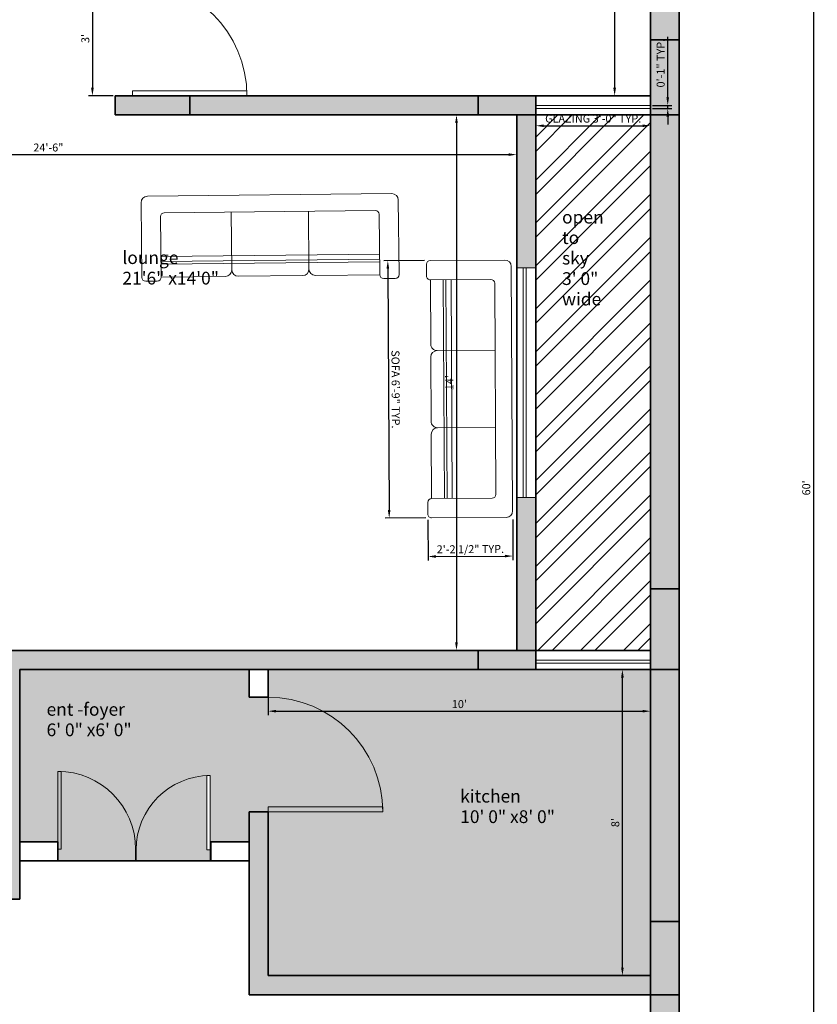
# Model space of a CAD drawing. Units: inches. Extents: x 2369 to 4208, y 1650 to 4492.
# Tile 4 of 6: x 2570 to 2820, y 1948 to 2257. Entities that reach past the tile are written whole.
import ezdxf

# ---------------------------------------------------------------- set-up
doc = ezdxf.new("R2010")
doc.units = ezdxf.units.IN
for name, color, linetype, lineweight in [('A-ANNO-DIMS', 2, 'Continuous', 13), ('A-AREA-IDEN', 7, 'Continuous', 18), ('A-COLS', 7, 'Continuous', 35), ('A-COLS-PATT', 7, 'Continuous', 13), ('A-DOOR', 4, 'Continuous', 18), ('A-FLOR-PATT', 9, 'Continuous', 13), ('A-FURN', 8, 'Continuous', 18), ('A-GLAZ', 4, 'Continuous', 18), ('A-WALL', 7, 'Continuous', 35), ('A-WALL-PATT', 252, 'Continuous', 13)]:
    doc.layers.add(name, color=color, linetype=linetype, lineweight=lineweight)
doc.styles.get("Standard").update_dxf_attribs({"font": 'arial.ttf'})
doc.dimstyles.new('Copy of ISO-25', dxfattribs={"dimtxt": 2.5, "dimasz": 2.5, "dimexe": 1.25, "dimexo": 0.625, "dimtad": 1, "dimdec": 1, "dimlunit": 4, "dimtxsty": 'Standard', "dimcen": 2.5, "dimadec": 0, "dimazin": 0, "dimtfac": 1, "dimtdec": 1, "dimtmove": 0, "dimatfit": 3, "dimfxl": 1, "dimarcsym": 0})

# ---------------------------------------------------------------- blocks, each defined once
blk = doc.blocks.new('*U5')
for p, q in [((0, 0), (0, -6)), ((-40, 0), (-40, -6))]:
    blk.add_line(p, q)
blk.add_lwpolyline([(0, 0), (0, 40), (-1.75, 40), (-1.75, 0)], close=True)
blk.add_arc((0, 0), 40, 90, 180)
blk = doc.blocks.new('*U4')
for p, q in [((-40, 0), (-40, 6)), ((0, 0), (0, 6))]:
    blk.add_line(p, q)
blk.add_lwpolyline([(0, 0), (0, -40), (-1.75, -40), (-1.75, 0)], close=True)
blk.add_arc((0, 0), 40, 180, 270)
blk = doc.blocks.new('*U2')
for p, q in [((0, 0), (0, -6)), ((40, 0), (40, -6))]:
    blk.add_line(p, q)
blk.add_lwpolyline([(0, 0), (0, 40), (1.75, 40), (1.75, 0)], close=True)
blk.add_arc((0, 0), 40, 0, 90)
blk = doc.blocks.new('*U3')
for p, q in [((0, 0), (0, -6)), ((-40, 0), (-40, -6))]:
    blk.add_line(p, q)
blk.add_lwpolyline([(0, 0), (0, 40), (-1.75, 40), (-1.75, 0)], close=True)
blk.add_arc((0, 0), 40, 90, 180)
blk = doc.blocks.new('*D8')
at = {"layer": 'A-ANNO-DIMS', "color": 0, "lineweight": -2, "transparency": 16777216}
for p, q in [((2777.53, 2469.98), (2820.25, 2469.98)), ((2819, 2467.48), (2819, 1752.48)), ((2777.53, 1749.98), (2820.25, 1749.98))]:
    blk.add_line(p, q, dxfattribs=at)
at = {"layer": 'A-ANNO-DIMS', "color": 0, "transparency": 16777216}
for points in [[(2818.58, 2467.48), (2819.41, 2467.48), (2819, 2469.98)], [(2818.58, 1752.48), (2819.41, 1752.48), (2819, 1749.98)]]:
    blk.add_solid(points, dxfattribs=at)
at = {"layer": 'Defpoints', "color": 0, "transparency": 16777216}
for p in [(2776.9, 2469.98), (2776.9, 1749.98), (2819, 1749.98)]:
    blk.add_point(p, dxfattribs=at)
at = {"layer": 'A-ANNO-DIMS', "color": 0, "transparency": 16777216, "insert": (2817.1, 2109.98), "char_height": 2.5, "attachment_point": 5, "rotation": 90}
blk.add_mtext("60'", dxfattribs=at)
blk = doc.blocks.new('*D22')
at = {"layer": 'A-ANNO-DIMS', "color": 0, "lineweight": -2, "transparency": 16777216}
for p, q in [((2767.28, 2394.98), (2755.38, 2394.98)), ((2756.63, 2392.48), (2756.63, 2235.48)), ((2767.28, 2232.98), (2755.38, 2232.98))]:
    blk.add_line(p, q, dxfattribs=at)
at = {"layer": 'A-ANNO-DIMS', "color": 0, "transparency": 16777216}
for points in [[(2756.21, 2392.48), (2757.05, 2392.48), (2756.63, 2394.98)], [(2756.21, 2235.48), (2757.05, 2235.48), (2756.63, 2232.98)]]:
    blk.add_solid(points, dxfattribs=at)
at = {"layer": 'Defpoints', "color": 0, "transparency": 16777216}
for p in [(2767.9, 2394.98), (2756.63, 2232.98), (2767.9, 2232.98)]:
    blk.add_point(p, dxfattribs=at)
at = {"layer": 'A-ANNO-DIMS', "color": 0, "transparency": 16777216, "insert": (2754.73, 2313.98), "char_height": 2.5, "attachment_point": 5, "rotation": 90}
blk.add_mtext('13\'-6"', dxfattribs=at)
blk = doc.blocks.new('*D27')
at = {"layer": 'A-ANNO-DIMS', "color": 0, "lineweight": -2, "transparency": 16777216}
for p, q in [((2431.9, 2226.35), (2431.9, 2213.28)), ((2725.9, 2226.35), (2725.9, 2213.28)), ((2434.4, 2214.53), (2723.4, 2214.53))]:
    blk.add_line(p, q, dxfattribs=at)
at = {"layer": 'A-ANNO-DIMS', "color": 0, "transparency": 16777216}
for points in [[(2434.4, 2214.94), (2434.4, 2214.11), (2431.9, 2214.53)], [(2723.4, 2214.94), (2723.4, 2214.11), (2725.9, 2214.53)]]:
    blk.add_solid(points, dxfattribs=at)
at = {"layer": 'Defpoints', "color": 0, "transparency": 16777216}
for p in [(2431.9, 2226.98), (2725.9, 2226.98), (2725.9, 2214.53)]:
    blk.add_point(p, dxfattribs=at)
at = {"layer": 'A-ANNO-DIMS', "color": 0, "transparency": 16777216, "insert": (2578.9, 2216.43), "char_height": 2.5, "attachment_point": 5}
blk.add_mtext('24\'-6"', dxfattribs=at)
blk = doc.blocks.new('*D28')
at = {"layer": 'A-ANNO-DIMS', "color": 0, "lineweight": -2, "transparency": 16777216}
for p, q in [((2725.28, 2226.98), (2705.75, 2226.98)), ((2707, 2224.48), (2707, 2061.48)), ((2725.28, 2058.98), (2705.75, 2058.98))]:
    blk.add_line(p, q, dxfattribs=at)
at = {"layer": 'A-ANNO-DIMS', "color": 0, "transparency": 16777216}
for points in [[(2706.58, 2224.48), (2707.41, 2224.48), (2707, 2226.98)], [(2706.58, 2061.48), (2707.41, 2061.48), (2707, 2058.98)]]:
    blk.add_solid(points, dxfattribs=at)
at = {"layer": 'Defpoints', "color": 0, "transparency": 16777216}
for p in [(2725.9, 2226.98), (2707, 2058.98), (2725.9, 2058.98)]:
    blk.add_point(p, dxfattribs=at)
at = {"layer": 'A-ANNO-DIMS', "color": 0, "transparency": 16777216, "insert": (2705.12, 2142.98), "char_height": 2.5, "attachment_point": 5, "rotation": 90}
blk.add_mtext("14'", dxfattribs=at)
blk = doc.blocks.new('*D31')
at = {"layer": 'A-ANNO-DIMS', "color": 0, "lineweight": -2, "transparency": 16777216}
for p, q in [((2647.9, 2052.35), (2647.9, 2038.68)), ((2767.9, 2052.35), (2767.9, 2038.68)), ((2650.4, 2039.93), (2765.4, 2039.93))]:
    blk.add_line(p, q, dxfattribs=at)
at = {"layer": 'A-ANNO-DIMS', "color": 0, "transparency": 16777216}
for points in [[(2650.4, 2040.34), (2650.4, 2039.51), (2647.9, 2039.93)], [(2765.4, 2040.34), (2765.4, 2039.51), (2767.9, 2039.93)]]:
    blk.add_solid(points, dxfattribs=at)
at = {"layer": 'Defpoints', "color": 0, "transparency": 16777216}
for p in [(2647.9, 2052.98), (2767.9, 2052.98), (2767.9, 2039.93)]:
    blk.add_point(p, dxfattribs=at)
at = {"layer": 'A-ANNO-DIMS', "color": 0, "transparency": 16777216, "insert": (2707.9, 2041.83), "char_height": 2.5, "attachment_point": 5}
blk.add_mtext("10'", dxfattribs=at)
blk = doc.blocks.new('*D32')
at = {"layer": 'A-ANNO-DIMS', "color": 0, "lineweight": -2, "transparency": 16777216}
for p, q in [((2767.28, 2052.98), (2757.82, 2052.98)), ((2759.07, 1959.48), (2759.07, 2050.48)), ((2767.28, 1956.98), (2757.82, 1956.98))]:
    blk.add_line(p, q, dxfattribs=at)
at = {"layer": 'A-ANNO-DIMS', "color": 0, "transparency": 16777216}
for points in [[(2758.66, 2050.48), (2759.49, 2050.48), (2759.07, 2052.98)], [(2758.66, 1959.48), (2759.49, 1959.48), (2759.07, 1956.98)]]:
    blk.add_solid(points, dxfattribs=at)
at = {"layer": 'Defpoints', "color": 0, "transparency": 16777216}
for p in [(2759.07, 2052.98), (2767.9, 2052.98), (2767.9, 1956.98)]:
    blk.add_point(p, dxfattribs=at)
at = {"layer": 'A-ANNO-DIMS', "color": 0, "transparency": 16777216, "insert": (2757.17, 2004.98), "char_height": 2.5, "attachment_point": 5, "rotation": 90}
blk.add_mtext("8'", dxfattribs=at)
blk = doc.blocks.new('*D43')
at = {"layer": 'A-ANNO-DIMS', "color": 0, "lineweight": -2, "transparency": 16777216}
for p, q in [((2599.28, 2268.93), (2591.48, 2268.93)), ((2592.73, 2266.43), (2592.73, 2235.48)), ((2599.28, 2232.98), (2591.48, 2232.98))]:
    blk.add_line(p, q, dxfattribs=at)
at = {"layer": 'A-ANNO-DIMS', "color": 0, "transparency": 16777216}
for points in [[(2592.31, 2266.43), (2593.15, 2266.43), (2592.73, 2268.93)], [(2592.31, 2235.48), (2593.15, 2235.48), (2592.73, 2232.98)]]:
    blk.add_solid(points, dxfattribs=at)
at = {"layer": 'Defpoints', "color": 0, "transparency": 16777216}
for p in [(2599.9, 2268.93), (2592.73, 2232.98), (2599.9, 2232.98)]:
    blk.add_point(p, dxfattribs=at)
at = {"layer": 'A-ANNO-DIMS', "color": 0, "transparency": 16777216, "insert": (2590.83, 2250.95), "char_height": 2.5, "attachment_point": 5, "rotation": 90}
blk.add_mtext("3'", dxfattribs=at)
blk = doc.blocks.new('A$C05BA3A2B')
for p, q in [((0.05, 0.6596), (1.95, 0.6596)), ((0.05, 0.6596), (1.95, 0.6596)), ((0.05, 0.6596), (1.95, 0.6596)), ((0, 0.03), (0, 0.6096)), ((0, 0.03), (0, 0.6096)), ((0, 0.03), (0, 0.6096)), ((2, 0.6096), (2, 0.03)), ((2, 0.6096), (2, 0.03)), ((2, 0.6096), (2, 0.03)), ((0.15, 0.5), (0.15, 0.03)), ((0.15, 0.5), (0.15, 0.03)), ((0.15, 0.5), (0.15, 0.03)), ((1.82, 0.53), (0.18, 0.53)), ((1.82, 0.53), (0.18, 0.53)), ((1.82, 0.53), (0.18, 0.53)), ((0.7, 0.08), (0.7, 0.53)), ((0.7, 0.08), (0.7, 0.53)), ((0.7, 0.08), (0.7, 0.53)), ((1.3, 0.53), (1.3, 0.08)), ((1.3, 0.53), (1.3, 0.08)), ((1.3, 0.53), (1.3, 0.08)), ((1.85, 0.03), (1.85, 0.5)), ((1.85, 0.03), (1.85, 0.5)), ((1.85, 0.03), (1.85, 0.5)), ((1.85, 0.1908), (0.15, 0.1908)), ((1.85, 0.1908), (0.15, 0.1908)), ((1.85, 0.1908), (0.15, 0.1908)), ((1.85, 0.1508), (0.15, 0.1508)), ((1.85, 0.1508), (0.15, 0.1508)), ((1.85, 0.1508), (0.15, 0.1508)), ((1.85, 0.1308), (0.15, 0.1308)), ((1.85, 0.1308), (0.15, 0.1308)), ((1.85, 0.1308), (0.15, 0.1308)), ((0.12, 0), (0.03, 0)), ((0.12, 0), (0.03, 0)), ((0.12, 0), (0.03, 0)), ((0.65, 0.03), (0.15, 0.03)), ((0.65, 0.03), (0.15, 0.03)), ((0.65, 0.03), (0.15, 0.03)), ((1.25, 0.03), (0.75, 0.03)), ((1.25, 0.03), (0.75, 0.03)), ((1.25, 0.03), (0.75, 0.03)), ((1.85, 0.03), (1.35, 0.03)), ((1.85, 0.03), (1.35, 0.03)), ((1.85, 0.03), (1.35, 0.03)), ((1.97, 0), (1.88, 0)), ((1.97, 0), (1.88, 0)), ((1.97, 0), (1.88, 0))]:
    blk.add_line(p, q)
for centre, radius, start, end in [((0.05, 0.6096), 0.05, 90, 180), ((0.05, 0.6096), 0.05, 90, 180), ((0.05, 0.6096), 0.05, 90, 180), ((1.95, 0.6096), 0.05, 0, 90), ((1.95, 0.6096), 0.05, 0, 90), ((1.95, 0.6096), 0.05, 0, 90), ((0.18, 0.5), 0.03, 90, 180), ((0.18, 0.5), 0.03, 90, 180), ((0.18, 0.5), 0.03, 90, 180), ((1.82, 0.5), 0.03, 0, 90), ((1.82, 0.5), 0.03, 0, 90), ((1.82, 0.5), 0.03, 0, 90), ((0.65, 0.08), 0.05, 270, 0), ((0.65, 0.08), 0.05, 270, 0), ((0.65, 0.08), 0.05, 270, 0), ((0.75, 0.08), 0.05, 180, 270), ((0.75, 0.08), 0.05, 180, 270), ((0.75, 0.08), 0.05, 180, 270), ((1.25, 0.08), 0.05, 270, 0), ((1.25, 0.08), 0.05, 270, 0), ((1.25, 0.08), 0.05, 270, 0), ((1.35, 0.08), 0.05, 180, 270), ((1.35, 0.08), 0.05, 180, 270), ((1.35, 0.08), 0.05, 180, 270), ((0.03, 0.03), 0.03, 180, 270), ((0.03, 0.03), 0.03, 180, 270), ((0.03, 0.03), 0.03, 180, 270), ((0.12, 0.03), 0.03, 270, 0), ((0.12, 0.03), 0.03, 270, 0), ((0.12, 0.03), 0.03, 270, 0), ((1.88, 0.03), 0.03, 180, 270), ((1.88, 0.03), 0.03, 180, 270), ((1.88, 0.03), 0.03, 180, 270), ((1.97, 0.03), 0.03, 270, 0), ((1.97, 0.03), 0.03, 270, 0), ((1.97, 0.03), 0.03, 270, 0)]:
    blk.add_arc(centre, radius, start, end)
blk = doc.blocks.new('GLAZING-36IN')
for p, q in [((0, 1), (36, 1)), ((0, 0), (36, 0))]:
    blk.add_line(p, q)
blk = doc.blocks.new('*D51')
at = {"layer": 'A-ANNO-DIMS', "color": 0, "lineweight": -2, "transparency": 16777216}
for p, q in [((2696.93, 2181.31), (2684.19, 2181.24)), ((2685.45, 2178.75), (2685.87, 2103)), ((2697.37, 2100.56), (2684.63, 2100.49))]:
    blk.add_line(p, q, dxfattribs=at)
at = {"layer": 'A-ANNO-DIMS', "color": 0, "transparency": 16777216}
for points in [[(2685.87, 2178.75), (2685.04, 2178.75), (2685.44, 2181.25)], [(2686.28, 2103), (2685.45, 2103), (2685.88, 2100.5)]]:
    blk.add_solid(points, dxfattribs=at)
at = {"layer": 'Defpoints', "color": 0, "transparency": 16777216}
for p in [(2697.55, 2181.32), (2685.88, 2100.5), (2697.99, 2100.57)]:
    blk.add_point(p, dxfattribs=at)
at = {"layer": 'A-ANNO-DIMS', "color": 0, "transparency": 16777216, "insert": (2687.58, 2140.89), "char_height": 2.5, "attachment_point": 5, "rotation": 270.3122}
blk.add_mtext('SOFA 6\'-9" TYP.', dxfattribs=at)
blk = doc.blocks.new('*D52')
at = {"layer": 'A-ANNO-DIMS', "color": 0, "lineweight": -2, "transparency": 16777216}
for p, q in [((2698, 2099.94), (2698.07, 2087.2)), ((2724.63, 2100.09), (2724.7, 2087.35)), ((2700.56, 2088.47), (2722.19, 2088.58))]:
    blk.add_line(p, q, dxfattribs=at)
at = {"layer": 'A-ANNO-DIMS', "color": 0, "transparency": 16777216}
for points in [[(2700.56, 2088.88), (2700.56, 2088.05), (2698.06, 2088.45)], [(2722.19, 2089), (2722.19, 2088.17), (2724.69, 2088.6)]]:
    blk.add_solid(points, dxfattribs=at)
at = {"layer": 'Defpoints', "color": 0, "transparency": 16777216}
for p in [(2697.99, 2100.57), (2724.62, 2100.71), (2724.69, 2088.6)]:
    blk.add_point(p, dxfattribs=at)
at = {"layer": 'A-ANNO-DIMS', "color": 0, "transparency": 16777216, "insert": (2711.36, 2090.44), "char_height": 2.5, "attachment_point": 5, "rotation": 0.3122}
blk.add_mtext('2\'-2 1/2" TYP.', dxfattribs=at)
blk = doc.blocks.new('*D53')
at = {"layer": 'A-ANNO-DIMS', "color": 0, "lineweight": -2, "transparency": 16777216}
for p, q in [((2731.9, 2228.35), (2731.9, 2222.33)), ((2767.9, 2228.35), (2767.9, 2222.33)), ((2734.4, 2223.58), (2765.4, 2223.58))]:
    blk.add_line(p, q, dxfattribs=at)
at = {"layer": 'A-ANNO-DIMS', "color": 0, "transparency": 16777216}
for points in [[(2734.4, 2224), (2734.4, 2223.16), (2731.9, 2223.58)], [(2765.4, 2224), (2765.4, 2223.16), (2767.9, 2223.58)]]:
    blk.add_solid(points, dxfattribs=at)
at = {"layer": 'Defpoints', "color": 0, "transparency": 16777216}
for p in [(2731.9, 2228.98), (2767.9, 2228.98), (2767.9, 2223.58)]:
    blk.add_point(p, dxfattribs=at)
at = {"layer": 'A-ANNO-DIMS', "color": 0, "transparency": 16777216, "insert": (2749.9, 2225.5), "char_height": 2.5, "attachment_point": 5}
blk.add_mtext('GLAZING 3\'-0" TYP.', dxfattribs=at)
blk = doc.blocks.new('*D54')
at = {"layer": 'A-ANNO-DIMS', "color": 0, "lineweight": -2, "transparency": 16777216}
for p, q in [((2773.3, 2232.48), (2773.3, 2251.47)), ((2768.53, 2229.98), (2774.55, 2229.98)), ((2768.53, 2228.98), (2774.55, 2228.98)), ((2773.3, 2228.98), (2773.3, 2229.98)), ((2773.3, 2226.48), (2773.3, 2223.98))]:
    blk.add_line(p, q, dxfattribs=at)
at = {"layer": 'A-ANNO-DIMS', "color": 0, "transparency": 16777216}
for points in [[(2772.88, 2232.48), (2773.72, 2232.48), (2773.3, 2229.98)], [(2772.88, 2226.48), (2773.72, 2226.48), (2773.3, 2228.98)]]:
    blk.add_solid(points, dxfattribs=at)
at = {"layer": 'Defpoints', "color": 0, "transparency": 16777216}
for p in [(2767.9, 2229.98), (2767.9, 2228.98), (2773.3, 2229.98)]:
    blk.add_point(p, dxfattribs=at)
at = {"layer": 'A-ANNO-DIMS', "color": 0, "transparency": 16777216, "insert": (2771.4, 2243.22), "char_height": 2.5, "attachment_point": 5, "rotation": 90}
blk.add_mtext('0\'-1" TYP.', dxfattribs=at)

msp = doc.modelspace()

# ---------------------------------------------------------------- hatches: boundary and pattern name
at = {"layer": 'A-COLS-PATT'}
h = msp.add_hatch(color=256, dxfattribs=at)
h.dxf.hatch_style = 1
h.paths.add_polyline_path([(2377.9, 2254.21), (2368.9, 2254.21), (2368.9, 2226.98), (2377.9, 2226.98)])
h.paths.add_polyline_path([(2551.9, 2400.98), (2545.9, 2400.98), (2525.15, 2400.98), (2525.15, 2394.98), (2545.9, 2395.12), (2551.9, 2395.12)])
h.paths.add_polyline_path([(2637.99, 2400.98), (2599.9, 2400.98), (2599.9, 2394.98), (2605.9, 2394.98), (2637.99, 2394.98)])
h.paths.add_polyline_path([(2623.27, 2232.98), (2599.9, 2232.98), (2599.9, 2226.98), (2623.27, 2226.98)])
h.paths.add_polyline_path([(2551.9, 2232.98), (2528.53, 2232.98), (2528.53, 2226.98), (2551.9, 2226.98)])
h.paths.add_polyline_path([(2731.9, 2232.98), (2713.81, 2232.98), (2713.81, 2226.98), (2731.9, 2226.98)])
h.paths.add_polyline_path([(2776.9, 2250.53), (2767.9, 2250.53), (2767.9, 2232.98), (2767.9, 2226.98), (2776.9, 2226.98)])
h.paths.add_polyline_path([(2776.9, 2078.3), (2767.9, 2078.3), (2767.9, 2058.98), (2767.9, 2052.98), (2776.9, 2052.98)])
h.paths.add_polyline_path([(2731.9, 2058.98), (2725.9, 2058.98), (2713.81, 2058.98), (2713.81, 2052.98), (2731.9, 2052.98)])
h.paths.add_polyline_path([(2776.9, 1973.96), (2767.9, 1973.96), (2767.9, 1956.98), (2767.9, 1950.98), (2776.9, 1950.98)])
h.paths.add_polyline_path([(2776.9, 1775.33), (2767.9, 1775.33), (2767.9, 1758.98), (2767.9, 1749.98), (2776.9, 1749.98)])
h.paths.add_polyline_path([(2569.9, 1758.98), (2560.9, 1758.98), (2560.9, 1749.98), (2569.9, 1749.98)])
h.paths.add_polyline_path([(2377.9, 1774.03), (2368.9, 1774.03), (2368.9, 1749.98), (2372.9, 1749.98), (2377.9, 1749.98)])
h.paths.add_polyline_path([(2377.9, 1926.53), (2368.9, 1926.53), (2368.9, 1902.98), (2377.9, 1902.98)])
h.paths.add_polyline_path([(2377.9, 2079.34), (2368.9, 2079.34), (2368.9, 2052.98), (2377.9, 2052.98), (2377.9, 2057.9)])
at = {"layer": 'A-FLOR-PATT'}
h = msp.add_hatch(dxfattribs=at)
h.set_pattern_fill('ANSI32', color=256)
h.paths.add_polyline_path([(2545.9, 2460.98), (2523.46, 2460.98), (2449.9, 2460.98), (2449.9, 2448.93, -0.401453), (2485.82, 2414.55), (2485.85, 2414.55), (2485.85, 2412.98), (2449.9, 2412.98), (2449.9, 2400.98), (2545.9, 2400.98)])
h.paths.add_polyline_path([(2701.9, 2448.92), (2701.9, 2460.98), (2605.9, 2460.98), (2605.9, 2400.98), (2637.99, 2400.98), (2701.9, 2400.98), (2701.9, 2412.98), (2666.56, 2412.98), (2666.56, 2414.55), (2666.59, 2414.55, -0.396556)])
h.paths.add_polyline_path([(2425.9, 2148.98), (2377.9, 2148.98), (2377.9, 2090.68), (2379.33, 2090.68), (2379.33, 2090.65, -0.391899), (2410.67, 2058.98), (2425.9, 2058.98), (2425.9, 2094.98), (2425.9, 2100.98)])
h.paths.add_polyline_path([(2401.9, 2460.98), (2377.9, 2460.98), (2377.9, 2400.98), (2401.9, 2400.98)])
h.paths.add_polyline_path([(2767.9, 2460.98), (2743.9, 2460.98), (2743.9, 2400.98), (2767.9, 2400.98)])
h.paths.add_polyline_path([(2767.9, 2226.98), (2731.9, 2226.98), (2731.9, 2058.98), (2767.9, 2058.98)])
h.paths.add_polyline_path([(2612.47, 2434.38), (2640.5, 2434.38), (2640.5, 2440.51), (2612.47, 2440.51)], flags=24)
h.paths.add_polyline_path([(2612.48, 2440.81), (2625.39, 2440.81), (2625.39, 2446.91), (2612.48, 2446.91)], flags=24)
h.paths.add_polyline_path([(2712.27, 2432.83), (2738.74, 2432.83), (2738.74, 2438.96), (2712.27, 2438.96)], flags=9)
h.paths.add_polyline_path([(2712.27, 2439.27), (2727.97, 2439.27), (2727.97, 2445.37), (2712.27, 2445.37)], flags=9)
h.paths.add_polyline_path([(2492.48, 2432.36), (2520.5, 2432.36), (2520.5, 2438.49), (2492.48, 2438.49)], flags=24)
h.paths.add_polyline_path([(2492.48, 2438.8), (2505.39, 2438.8), (2505.39, 2444.9), (2492.48, 2444.9)], flags=24)
h.paths.add_polyline_path([(2386, 2119.22), (2414.03, 2119.22), (2414.03, 2125.35), (2386, 2125.35)], flags=24)
h.paths.add_polyline_path([(2386.01, 2125.66), (2398.92, 2125.66), (2398.92, 2131.75), (2386.01, 2131.75)], flags=24)
h.paths.add_polyline_path([(2377.88, 2440.75), (2403.21, 2440.75), (2403.21, 2446.85), (2377.88, 2446.85)], flags=9)
h.paths.add_polyline_path([(2743.66, 2441.21), (2768.99, 2441.21), (2768.99, 2447.31), (2743.66, 2447.31)], flags=9)
h.paths.add_polyline_path([(2739.13, 2166.12), (2752.65, 2166.12), (2752.65, 2172.22), (2739.13, 2172.22)], flags=24)
h.paths.add_polyline_path([(2739.12, 2172.54), (2751.98, 2172.54), (2751.98, 2178.67), (2739.12, 2178.67)], flags=24)
h.paths.add_polyline_path([(2738.85, 2177.59), (2749.82, 2177.59), (2749.82, 2185.35), (2738.85, 2185.35)], flags=24)
h.paths.add_polyline_path([(2739.15, 2185.42), (2747.35, 2185.42), (2747.35, 2191.39), (2739.15, 2191.39)], flags=24)
h.paths.add_polyline_path([(2739.12, 2190.78), (2753.59, 2190.78), (2753.59, 2196.89), (2739.12, 2196.89)], flags=24)
h = msp.add_hatch(dxfattribs=at)
h.set_pattern_fill('ANGLE', color=256)
h.set_pattern_definition([(0, (0, 0), (0, 6.985), [5.08, -1.905]), (90, (0, 0), (-6.985, 4e-16), [5.08, -1.905])])
h.paths.add_polyline_path([(2599.9, 2460.98), (2551.9, 2460.98), (2551.9, 2298.98), (2563.9, 2298.98), (2563.9, 2306.63), (2564.42, 2306.63), (2564.42, 2306.61, -0.405418), (2575.94, 2294.77, -0.401619), (2587.38, 2306.72), (2587.38, 2306.73), (2587.9, 2306.73), (2587.9, 2298.98), (2599.9, 2298.98)])
h.paths.add_polyline_path([(2425.9, 2226.98), (2377.9, 2226.98), (2377.9, 2154.98), (2389.9, 2154.98), (2425.9, 2154.98)])
h.paths.add_polyline_path([(2641.9, 2052.98), (2569.9, 2052.98), (2569.9, 1998.98), (2581.9, 1998.98), (2581.9, 1992.98), (2606.44, 1992.98), (2629.9, 1992.98), (2629.9, 1998.98), (2641.9, 1998.98), (2641.9, 2008.36), (2647.9, 2008.36), (2647.9, 1956.98), (2767.9, 1956.98), (2767.9, 2052.98), (2647.9, 2052.98), (2647.9, 2044.36), (2641.9, 2044.36)])
h.paths.add_polyline_path([(2628.69, 2019.73), (2629.71, 2019.73), (2629.71, 1996.47), (2628.69, 1996.47)], flags=16)
h.paths.add_polyline_path([(2563.51, 2406.86), (2576.05, 2406.86), (2576.05, 2412.82), (2563.51, 2412.82)], flags=24)
h.paths.add_polyline_path([(2391.33, 2190.25), (2403.87, 2190.25), (2403.87, 2196.21), (2391.33, 2196.21)], flags=24)
h.paths.add_polyline_path([(2704.89, 2039.23), (2710.69, 2039.23), (2710.69, 2044.38), (2704.89, 2044.38)], flags=24)
h.paths.add_polyline_path([(2759.77, 2003.06), (2759.77, 2006.92), (2754.62, 2006.92), (2754.62, 2003.06)], flags=24)
h.paths.add_polyline_path([(2707.15, 2003.75), (2738.28, 2003.75), (2738.28, 2009.88), (2707.15, 2009.88)], flags=24)
h.paths.add_polyline_path([(2707.15, 2010.19), (2726.89, 2010.19), (2726.89, 2016.29), (2707.15, 2016.29)], flags=24)
h.paths.add_polyline_path([(2577.31, 2031), (2605.34, 2031), (2605.34, 2037.12), (2577.31, 2037.12)], flags=24)
h.paths.add_polyline_path([(2577.02, 2036.02), (2603.33, 2036.02), (2603.33, 2043.89), (2577.02, 2043.89)], flags=24)
at = {"layer": 'A-WALL-PATT'}
h = msp.add_hatch(color=256, dxfattribs=at)
h.dxf.hatch_style = 1
h.paths.add_polyline_path([(2377.9, 2052.98), (2368.9, 2052.98), (2368.9, 1926.53), (2377.9, 1926.53)])
h.paths.add_polyline_path([(2377.9, 2226.98), (2368.9, 2226.98), (2368.9, 2079.34), (2377.9, 2079.34)])
h.paths.add_polyline_path([(2377.9, 2394.98), (2377.9, 2460.98), (2767.9, 2460.98), (2767.9, 2250.53), (2776.9, 2250.53), (2776.9, 2469.98), (2368.9, 2469.98), (2368.9, 2254.21), (2377.9, 2254.21)])
h.paths.add_polyline_path([(2776.9, 2226.98), (2767.9, 2226.98), (2767.9, 2078.3), (2776.9, 2078.3)])
h.paths.add_polyline_path([(2776.9, 2052.98), (2767.9, 2052.98), (2767.9, 1973.96), (2776.9, 1973.96)])
h.paths.add_polyline_path([(2776.9, 1950.98), (2767.9, 1950.98), (2767.9, 1775.33), (2776.9, 1775.33)])
h.paths.add_polyline_path([(2560.9, 1758.98), (2377.9, 1758.98), (2377.9, 1749.98), (2386.24, 1749.98), (2386.07, 1750.89), (2387.22, 1749.98), (2560.9, 1749.98)])
h.paths.add_polyline_path([(2377.9, 1902.98), (2368.9, 1902.98), (2368.9, 1774.03), (2377.9, 1774.03)])
h.paths.add_polyline_path([(2569.9, 1908.98), (2569.9, 1944.98), (2563.9, 1944.98), (2563.9, 1908.98), (2377.9, 1908.98), (2377.9, 1902.98), (2569.9, 1902.98)])
h.paths.add_polyline_path([(2523.29, 2058.98), (2411, 2058.98), (2411, 2052.98), (2523.29, 2052.98)])
h.paths.add_polyline_path([(2569.9, 2052.98), (2641.9, 2052.98), (2713.81, 2052.98), (2713.81, 2058.98), (2559.29, 2058.98), (2559.29, 2052.98), (2563.9, 2052.98), (2563.9, 1980.98), (2569.9, 1980.98), (2569.9, 1992.98)])
h.paths.add_polyline_path([(2528.53, 2232.98), (2510.56, 2232.98), (2377.9, 2232.98), (2377.9, 2226.98), (2528.53, 2226.98)])
h.paths.add_polyline_path([(2713.81, 2232.98), (2623.27, 2232.98), (2623.27, 2226.98), (2713.81, 2226.98)])
h.paths.add_polyline_path([(2647.9, 2008.36), (2642.51, 2008.36), (2641.9, 2008.36), (2641.9, 1956.98), (2641.9, 1950.98), (2767.9, 1950.98), (2767.9, 1956.98), (2647.9, 1956.98)])
h.paths.add_polyline_path([(2551.9, 2395.12), (2545.9, 2395.12), (2545.9, 2268.98), (2551.9, 2268.98)], flags=17)
h.paths.add_polyline_path([(2551.9, 2460.98), (2545.9, 2460.98), (2545.9, 2400.98), (2551.9, 2400.98)], flags=17)
h.paths.add_polyline_path([(2605.9, 2460.98), (2599.9, 2460.98), (2599.9, 2400.98), (2605.9, 2400.98)], flags=17)
h.paths.add_polyline_path([(2767.9, 2400.98), (2637.99, 2400.98), (2637.99, 2394.98), (2767.9, 2394.98)], flags=17)
h.paths.add_polyline_path([(2605.9, 2394.98), (2599.9, 2394.98), (2599.9, 2394.42), (2599.9, 2268.98), (2605.9, 2268.98)], flags=17)
h.paths.add_polyline_path([(2525.15, 2400.98), (2377.9, 2400.98), (2377.9, 2394.98), (2525.15, 2394.98)], flags=17)
h.paths.add_polyline_path([(2449.9, 2412.98), (2444.51, 2412.98), (2443.9, 2412.98), (2443.9, 2400.98), (2449.9, 2400.98)], flags=17)
h.paths.add_polyline_path([(2449.9, 2460.98), (2443.9, 2460.98), (2443.9, 2448.98), (2449.9, 2448.98)], flags=17)
h.paths.add_polyline_path([(2731.9, 2106.98), (2725.9, 2106.98), (2725.9, 2058.98), (2731.9, 2058.98)])
h = msp.add_hatch(color=256, dxfattribs=at)
h.dxf.hatch_style = 1
h.paths.add_polyline_path([(2731.9, 2226.98), (2725.9, 2226.98), (2725.9, 2178.98), (2731.9, 2178.98)])

# ---------------------------------------------------------------- linework, layer by layer
at = {"layer": 'A-COLS'}
for p, q in [((2776.9, 2250.53), (2767.9, 2250.53)), ((2776.9, 2226.98), (2776.9, 2250.53)), ((2599.9, 2232.98), (2599.9, 2226.98)), ((2599.9, 2232.98), (2623.27, 2232.98)), ((2623.27, 2232.98), (2623.27, 2226.98)), ((2713.81, 2226.98), (2713.81, 2232.98)), ((2731.9, 2226.98), (2731.9, 2232.98)), ((2767.9, 2226.98), (2767.9, 2232.98)), ((2767.9, 2226.98), (2776.9, 2226.98)), ((2776.9, 2078.3), (2767.9, 2078.3)), ((2776.9, 2052.98), (2776.9, 2078.3)), ((2725.9, 2058.98), (2713.81, 2058.98)), ((2713.81, 2058.98), (2713.81, 2052.98)), ((2731.9, 2058.98), (2731.9, 2052.98)), ((2767.9, 2058.98), (2767.9, 2052.98)), ((2767.9, 2052.98), (2776.9, 2052.98)), ((2776.9, 1973.96), (2767.9, 1973.96)), ((2776.9, 1950.98), (2776.9, 1973.96)), ((2767.9, 1950.98), (2776.9, 1950.98))]:
    msp.add_line(p, q, dxfattribs=at)
at = {"layer": 'A-DOOR'}
msp.add_line((2581.9, 1992.98), (2606.44, 1992.98), dxfattribs=at)
at = {"layer": 'A-GLAZ'}
for p, q in [((2725.9, 2178.98), (2731.9, 2178.98)), ((2727.9, 2178.98), (2727.9, 2106.98)), ((2728.9, 2178.98), (2728.9, 2106.98)), ((2731.9, 2178.98), (2731.9, 2106.98)), ((2731.9, 2106.98), (2725.9, 2106.98))]:
    msp.add_line(p, q, dxfattribs=at)
at = {"layer": 'A-WALL'}
for p, q in [((2767.9, 2232.98), (2599.9, 2232.98)), ((2599.9, 2226.98), (2767.9, 2226.98)), ((2725.9, 2058.98), (2725.9, 2226.98)), ((2725.9, 2226.98), (2725.9, 2178.98)), ((2767.9, 2226.98), (2731.9, 2226.98)), ((2731.9, 2226.98), (2731.9, 2058.98)), ((2767.9, 2226.98), (2767.9, 2058.98)), ((2767.9, 2058.98), (2559.29, 2058.98)), ((2563.9, 2058.98), (2570.14, 2058.98)), ((2731.9, 2058.98), (2725.9, 2058.98)), ((2641.9, 2052.98), (2569.9, 2052.98)), ((2569.9, 2052.98), (2569.9, 1980.98)), ((2569.9, 2052.98), (2767.9, 2052.98)), ((2647.9, 2052.98), (2641.9, 2052.98)), ((2641.9, 2052.98), (2641.9, 2044.36)), ((2641.9, 2052.98), (2641.9, 2044.36)), ((2647.9, 2044.36), (2647.9, 2052.98)), ((2647.9, 2044.36), (2647.9, 2052.98)), ((2767.9, 2052.98), (2767.9, 1956.98)), ((2641.9, 2044.36), (2647.9, 2044.36)), ((2647.9, 2008.36), (2641.9, 2008.36)), ((2641.9, 2008.36), (2641.9, 1956.98)), ((2647.9, 1956.98), (2647.9, 2008.36)), ((2581.9, 1998.98), (2569.9, 1998.98)), ((2581.9, 1992.98), (2581.9, 1998.98)), ((2641.9, 1998.98), (2629.9, 1998.98)), ((2629.9, 1998.98), (2629.9, 1992.98)), ((2641.9, 1992.98), (2641.9, 1998.98)), ((2569.9, 1980.98), (2569.9, 1992.98)), ((2569.9, 1992.98), (2581.9, 1992.98)), ((2581.9, 1992.98), (2641.9, 1992.98)), ((2569.9, 1980.98), (2563.9, 1980.98)), ((2641.9, 1956.98), (2641.9, 1950.98)), ((2767.9, 1956.98), (2647.9, 1956.98)), ((2641.9, 1950.98), (2767.9, 1950.98))]:
    msp.add_line(p, q, dxfattribs=at)
for points in [[(2368.9, 1749.98), (2368.9, 2469.98), (2776.9, 2469.98), (2776.9, 1749.98), (2689.9, 1749.98)], [(2767.9, 2052.98), (2767.9, 1758.98), (2377.9, 1758.98), (2377.9, 2460.98), (2767.9, 2460.98), (2767.9, 2232.98)], [(2767.9, 2226.98), (2767.9, 2058.98)]]:
    msp.add_lwpolyline(points, dxfattribs=at)

# ---------------------------------------------------------------- block references
at = {"layer": 'A-DOOR', "xscale": 0.8987594980764617, "yscale": 0.8987594980764617, "zscale": 0.8987594980764617, "rotation": 270}
for name, p in [('*U5', (2605.29, 2232.98)), ('*U5', (2647.9, 2008.36)), ('*U4', (2564.51, 1944.98))]:
    msp.add_blockref(name, p, dxfattribs=at)
at = {"layer": 'A-DOOR'}
for name, p, xscale, yscale, zscale in [('*U2', (2581.9, 1996.64), 0.6098804071616929, 0.6098804071616929, 0.6098804071616929), ('*U3', (2629.71, 1996.47), 0.5816555649327863, 0.5816555649327863, 0.5816555649327863)]:
    msp.add_blockref(name, p, dxfattribs=dict(at, xscale=xscale, yscale=yscale, zscale=zscale))
at = {"layer": 'A-FURN', "xscale": 40.37667945579769, "yscale": 40.37667945579769, "zscale": 40.37667945579769}
for p, rotation in [((2608.25, 2174.81), 0.6244003852997521), ((2697.55, 2181.32), 270.3122001926737)]:
    msp.add_blockref('A$C05BA3A2B', p, dxfattribs=dict(at, rotation=rotation))
at = {"layer": 'A-GLAZ'}
msp.add_blockref('GLAZING-36IN', (2731.9, 2228.98), dxfattribs=at)
at = {"layer": 'A-GLAZ', "rotation": 180}
msp.add_blockref('GLAZING-36IN', (2767.9, 2055.98), dxfattribs=at)

# ---------------------------------------------------------------- texts
at = {"layer": 'A-AREA-IDEN'}
for s, p in [('open', (2740.14, 2192.91)), ('to ', (2740.14, 2186.48)), ('lounge', (2602.13, 2180.21)), ('sky', (2740.14, 2180.06)), ('21\'6" x14\'0"', (2602.13, 2173.78)), ('3\' 0"', (2740.14, 2173.63)), ('wide', (2740.14, 2167.21)), ('ent -foyer', (2578.34, 2038.51)), ('6\' 0" x6\' 0"', (2578.34, 2032.08)), ('kitchen', (2708.17, 2011.27)), ('10\' 0" x8\' 0"', (2708.17, 2004.84))]:
    msp.add_text(s, height=4, dxfattribs=at).set_placement(p)

# ---------------------------------------------------------------- dimensions: what is measured, and where the dimension line sits
at = {"layer": 'A-ANNO-DIMS'}
for base, p1, p2, picture, middle in [((2819, 1749.98), (2776.9, 2469.98), (2776.9, 1749.98), '*D8', (2817.1, 2109.98)), ((2756.63, 2232.98), (2767.9, 2394.98), (2767.9, 2232.98), '*D22', (2754.73, 2313.98)), ((2592.7288, 2232.9785), (2599.9004, 2268.9289), (2599.9004, 2232.9785), '*D43', (2590.8265, 2250.9537)), ((2707, 2058.98), (2725.9, 2226.98), (2725.9, 2058.98), '*D28', (2705.12, 2142.98)), ((2759.07, 2052.98), (2767.9, 1956.98), (2767.9, 2052.98), '*D32', (2757.17, 2004.98))]:
    dim = msp.add_linear_dim(base=base, p1=p1, p2=p2, angle=90, dimstyle='Copy of ISO-25', override={"dimclrd": 0, "dimclre": 0, "dimclrt": 0}, dxfattribs=at)
    dim.commit()
    dim.dimension.update_dxf_attribs({"geometry": picture, "text_midpoint": middle})
for base, p1, p2, angle, text, picture, middle in [((2773.3, 2229.98), (2767.9, 2228.98), (2767.9, 2229.98), 90, '<> TYP.', '*D54', (2771.4, 2243.22)), ((2685.88, 2100.5), (2697.55, 2181.32), (2697.99, 2100.57), 270.3122, 'SOFA <> TYP.', '*D51', (2687.58, 2140.89)), ((2724.69, 2088.6), (2697.99, 2100.57), (2724.62, 2100.71), 0.3122, '<> TYP.', '*D52', (2711.36, 2090.44))]:
    dim = msp.add_linear_dim(base=base, p1=p1, p2=p2, angle=angle, text=text, dimstyle='Copy of ISO-25', override={"dimdec": 1, "dimlfac": 1, "dimrnd": 0, "dimzin": 1, "dimdsep": 46, "dimlunit": 4, "dimfrac": 2}, dxfattribs=at)
    dim.commit()
    dim.dimension.update_dxf_attribs({"geometry": picture, "text_midpoint": middle})
dim = msp.add_linear_dim(base=(2767.9, 2223.58), p1=(2731.9, 2228.98), p2=(2767.9, 2228.98), text='GLAZING <> TYP.', dimstyle='Copy of ISO-25', override={"dimdec": 1, "dimlfac": 1, "dimrnd": 0, "dimzin": 1, "dimdsep": 46, "dimlunit": 4, "dimfrac": 2}, dxfattribs=at)
dim.commit()
dim.dimension.update_dxf_attribs({"geometry": '*D53', "text_midpoint": (2749.9, 2225.5)})
for base, p1, p2, picture, middle in [((2725.9, 2214.53), (2431.9, 2226.98), (2725.9, 2226.98), '*D27', (2578.9, 2216.43)), ((2767.9, 2039.93), (2647.9, 2052.98), (2767.9, 2052.98), '*D31', (2707.9, 2041.83))]:
    dim = msp.add_linear_dim(base=base, p1=p1, p2=p2, dimstyle='Copy of ISO-25', override={"dimclrd": 0, "dimclre": 0, "dimclrt": 0}, dxfattribs=at)
    dim.commit()
    dim.dimension.update_dxf_attribs({"geometry": picture, "text_midpoint": middle})

doc.saveas('drawing.dxf')
